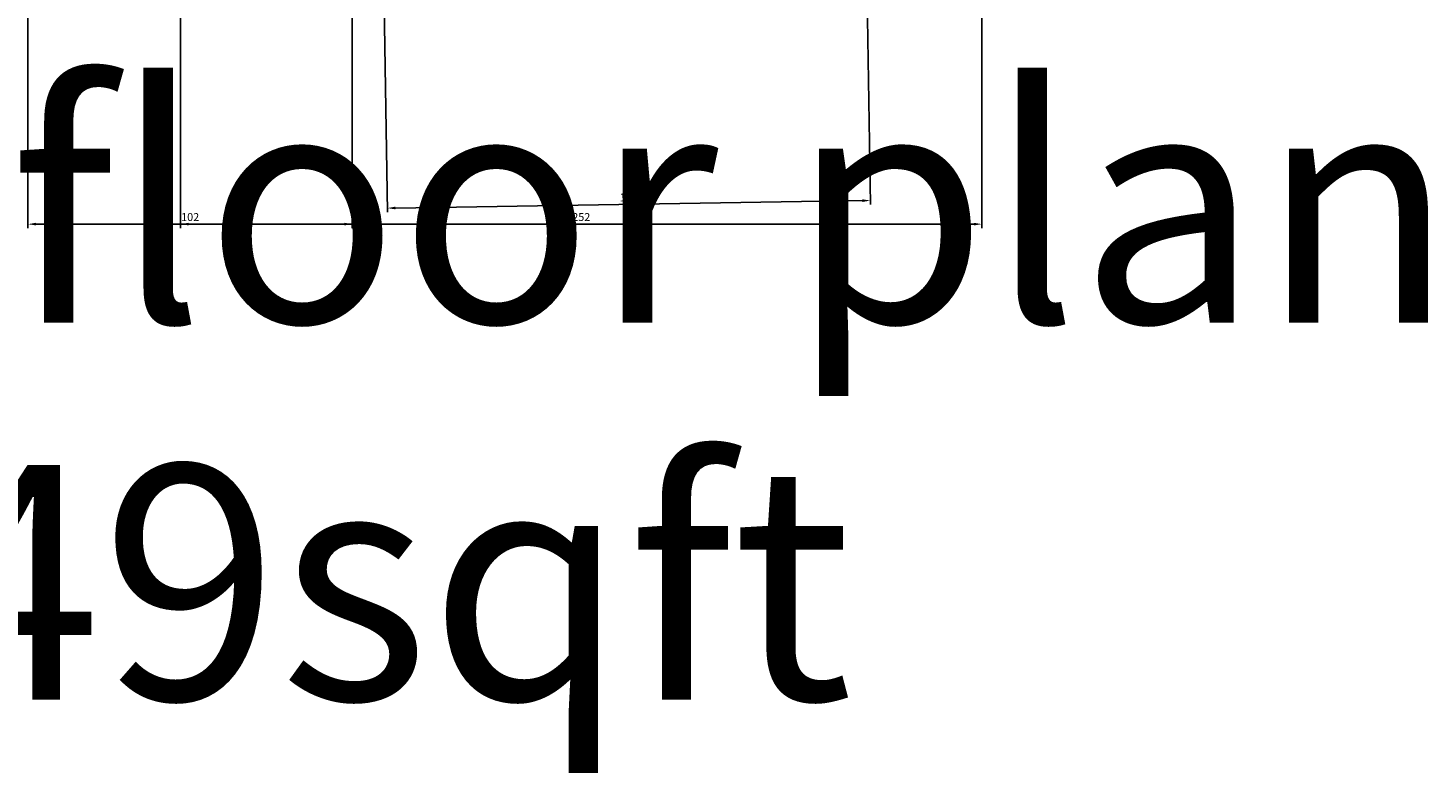
# Model space of a CAD drawing. Units: inches. Extents: x 604 to 3492, y -123 to 1737.
# Tile 3 of 20: x 1038 to 1478, y -104 to 131. Entities that reach past the tile are written whole.
import ezdxf

# ---------------------------------------------------------------- set-up
doc = ezdxf.new("R2010")
doc.units = ezdxf.units.IN
for name, color, linetype, lineweight in [('A-ANNO-DIMS', 2, 'Continuous', 18), ('A-ANNO-TEXT', 7, 'Continuous', 35), ('A-AREA-IDEN', 7, 'Continuous', 25)]:
    doc.layers.add(name, color=color, linetype=linetype, lineweight=lineweight)
doc.styles.get("Standard").update_dxf_attribs({"font": 'arial.ttf'})
doc.dimstyles.new('ISO-25', dxfattribs={"dimtxt": 2.5, "dimasz": 2.5, "dimexe": 1.25, "dimexo": 0.625, "dimtad": 1, "dimtxsty": 'Standard', "dimcen": 2.5, "dimadec": 0, "dimazin": 0, "dimtfac": 1, "dimtmove": 0, "dimatfit": 3, "dimfxl": 1, "dimarcsym": 0})

# ---------------------------------------------------------------- blocks, each defined once
blk = doc.blocks.new('*D82')
at = {"layer": 'A-ANNO-DIMS', "color": 0, "lineweight": -2, "transparency": 16777216}
for p, q in [((1150.03, 138), (1151.06, 72.81)), ((1301.94, 140.38), (1302.96, 75.2)), ((1153.54, 74.1), (1300.44, 76.41))]:
    blk.add_line(p, q, dxfattribs=at)
at = {"layer": 'A-ANNO-DIMS', "color": 0, "transparency": 16777216}
for points in [[(1300.44, 76.83), (1300.45, 76), (1302.94, 76.45)], [(1153.53, 74.52), (1153.54, 73.69), (1151.04, 74.06)]]:
    blk.add_solid(points, dxfattribs=at)
at = {"layer": 'Defpoints', "color": 0, "transparency": 16777216}
for p in [(1301.93, 141.01), (1150.02, 138.62), (1302.94, 76.45)]:
    blk.add_point(p, dxfattribs=at)
at = {"layer": 'A-ANNO-DIMS', "color": 0, "transparency": 16777216, "insert": (1226.96, 77.16), "char_height": 2.5, "attachment_point": 5, "rotation": 0.9007}
blk.add_mtext('152', dxfattribs=at)
blk = doc.blocks.new('*D86')
at = {"layer": 'A-ANNO-DIMS', "color": 0, "lineweight": -2, "transparency": 16777216}
for p, q in [((1038.01, 1272.08), (1038.01, 67.77)), ((1140.01, 1272.08), (1140.01, 67.77)), ((1040.51, 69.02), (1137.51, 69.02))]:
    blk.add_line(p, q, dxfattribs=at)
at = {"layer": 'A-ANNO-DIMS', "color": 0, "transparency": 16777216}
for points in [[(1040.51, 69.44), (1040.51, 68.61), (1038.01, 69.02)], [(1137.51, 69.44), (1137.51, 68.61), (1140.01, 69.02)]]:
    blk.add_solid(points, dxfattribs=at)
at = {"layer": 'Defpoints', "color": 0, "transparency": 16777216}
for p in [(1038.01, 1272.7), (1140.01, 1272.7), (1140.01, 69.02)]:
    blk.add_point(p, dxfattribs=at)
at = {"layer": 'A-ANNO-DIMS', "color": 0, "transparency": 16777216, "insert": (1089.01, 70.93), "char_height": 2.5, "attachment_point": 5}
blk.add_mtext('102', dxfattribs=at)
blk = doc.blocks.new('*D94')
at = {"layer": 'A-ANNO-DIMS', "color": 0, "lineweight": -2, "transparency": 16777216}
for p, q in [((1086.01, 602.08), (1086.01, 67.77)), ((1338.01, 602.08), (1338.01, 67.77)), ((1088.51, 69.02), (1335.51, 69.02))]:
    blk.add_line(p, q, dxfattribs=at)
at = {"layer": 'A-ANNO-DIMS', "color": 0, "transparency": 16777216}
for points in [[(1088.51, 69.44), (1088.51, 68.61), (1086.01, 69.02)], [(1335.51, 69.44), (1335.51, 68.61), (1338.01, 69.02)]]:
    blk.add_solid(points, dxfattribs=at)
at = {"layer": 'Defpoints', "color": 0, "transparency": 16777216}
for p in [(1086.01, 602.7), (1338.01, 602.7), (1338.01, 69.02)]:
    blk.add_point(p, dxfattribs=at)
at = {"layer": 'A-ANNO-DIMS', "color": 0, "transparency": 16777216, "insert": (1212.01, 70.93), "char_height": 2.5, "attachment_point": 5}
blk.add_mtext('252', dxfattribs=at)

msp = doc.modelspace()

# ---------------------------------------------------------------- texts
at = {"layer": 'A-ANNO-TEXT'}
msp.add_text('ground floor plan', height=73.861865, dxfattribs=at).set_placement((667.6364, 38.0072))
at = {"layer": 'A-AREA-IDEN'}
msp.add_text('area : 749sqft', height=73.861865, dxfattribs=at).set_placement((667.6364, -80.6454))

# ---------------------------------------------------------------- dimensions: what is measured, and where the dimension line sits
at = {"layer": 'A-ANNO-DIMS'}
for base, p1, p2, picture, middle in [((1140.0111, 69.0242), (1038.0111, 1272.7004), (1140.0111, 1272.7004), '*D86', (1089.0111, 70.9256)), ((1338.0111, 69.0242), (1086.0111, 602.7004), (1338.0111, 602.7004), '*D94', (1212.0111, 70.9256))]:
    dim = msp.add_linear_dim(base=base, p1=p1, p2=p2, dimstyle='ISO-25', override={"dimdec": 0, "dimlfac": 1, "dimrnd": 0, "dimzin": 0, "dimdsep": 46, "dimlunit": 2}, dxfattribs=at)
    dim.commit()
    dim.dimension.update_dxf_attribs({"geometry": picture, "text_midpoint": middle})
dim = msp.add_linear_dim(base=(1302.9429, 76.4518), p1=(1150.0221, 138.6204), p2=(1301.9279, 141.0087), angle=0.900725, dimstyle='ISO-25', override={"dimdec": 0, "dimlfac": 1, "dimrnd": 0, "dimzin": 0, "dimdsep": 46, "dimlunit": 2}, dxfattribs=at)
dim.commit()
dim.dimension.update_dxf_attribs({"geometry": '*D82', "text_midpoint": (1226.9601, 77.1589)})

doc.saveas('drawing.dxf')
